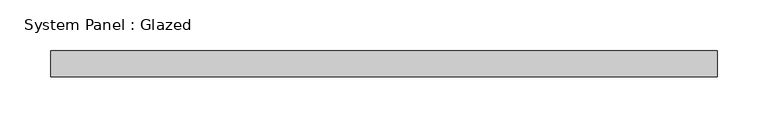
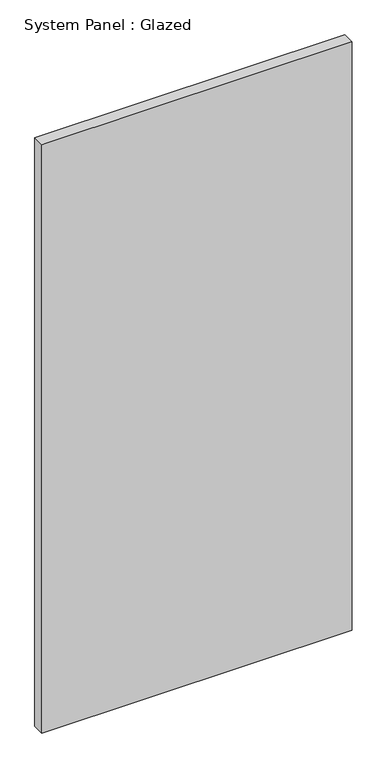
"""IFC4 building model written with IfcOpenShell, lengths in millimetres: plate geometry, System Panel : Glazed."""

from ifc_helpers import new_model, si_unit, origin, origin_with_axes, place, context, project, spatial, polyline, outline, extrude, source, transform, mapped, element, save


def system_panel_glazed_82e5a723(model_context):
    return source(origin(), model_context, "Body", "SweptSolid", [
        extrude(outline(polyline([(328.0833333, 19.05), (-328.0833333, 19.05), (-328.0833333, 44.45), (328.0833333, 44.45), (328.0833333, 19.05)])), origin_with_axes(), (0.0, 0.0, 1.0), 1315.3193903),
    ])


if __name__ == "__main__":
    model = new_model("IFC4")
    model_context = context("Model", 3, world=origin())
    ifc_project = project(units=[si_unit("LENGTHUNIT", "METRE", prefix="MILLI")], contexts=[model_context])
    site = spatial("IfcSite", under=ifc_project)
    building = spatial("IfcBuilding", under=site)
    placement = place(None, origin())
    system_panel_glazed_shape = system_panel_glazed_82e5a723(model_context)
    element("IfcPlate", 1, ObjectType="System Panel : Glazed", at=placement, inside=building, context=model_context, shape_type="MappedRepresentation", body=[
        mapped(system_panel_glazed_shape, transform((0.0, 0.0, 0.0), x_axis=(1.0, 0.0, 0.0), y_axis=(0.0, 1.0, 0.0), z_axis=(0.0, 0.0, 1.0))),
    ])
    save(model, "model.ifc")

# Revit data of these elements
# Type "System Panel : Glazed"
#   Construction Type Id = "GSP4R"
#   Analytic Construction = "1/8 in Pilkington single glazing"
#   Visual Light Transmittance = 0.9
#   Solar Heat Gain Coefficient = 0.86
#   Heat Transfer Coefficient (U) = 1.18115 BTU/(h·ft²·°F)
#   Define Thermal Properties by = 1
# Element 1 (IfcPlate, "System Panel : Glazed")
#   Materials on its faces: "Glass"
# Materials
#   "Glass": class "Glass", colour RGB 0 128 192, transparency 0.75, Description = "Soda Lime Glass", Cost = 0
